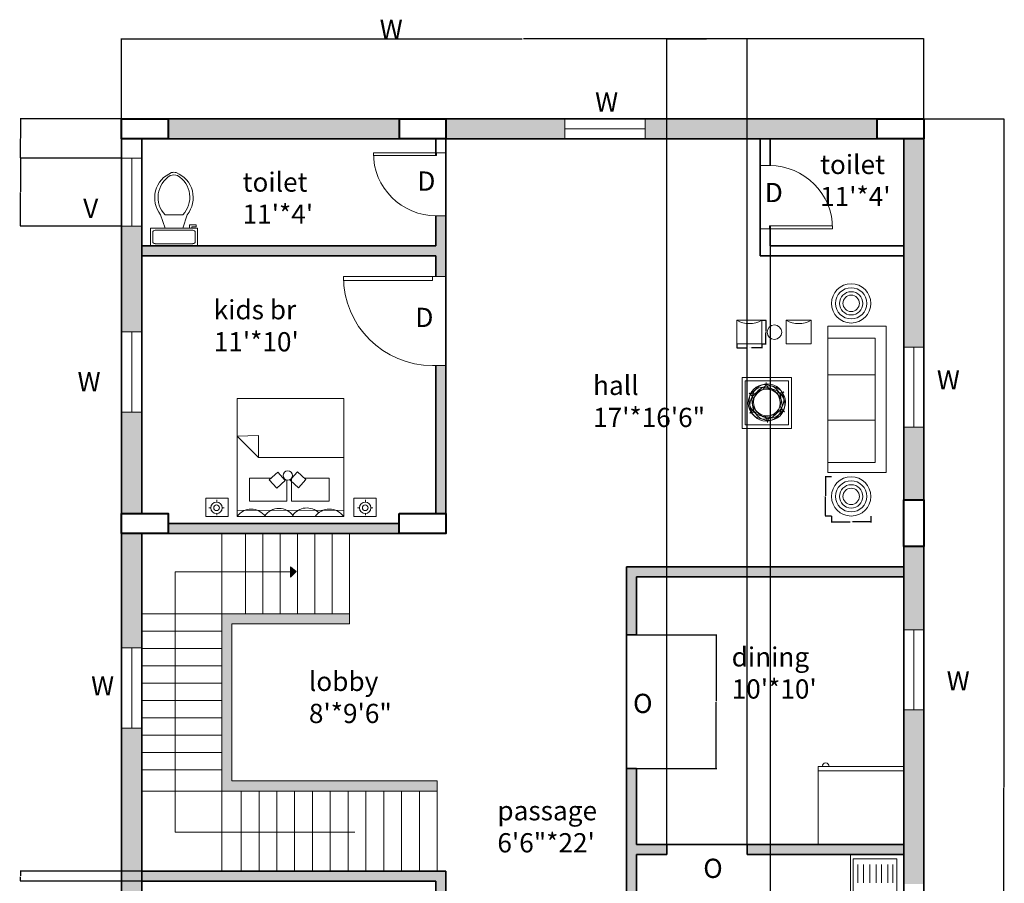
# Model space of a CAD drawing. Units: inches. Extents: x 1568 to 2529, y 2149 to 2897.
# Tile 13 of 16: x 1568 to 2010, y 2459 to 2846. Entities that reach past the tile are written whole.
import ezdxf

# ---------------------------------------------------------------- set-up
doc = ezdxf.new("R2010")
doc.units = ezdxf.units.IN
for name, color, linetype, lineweight in [('A-ANNO-DIMS', 2, 'Continuous', 18), ('A-ANNO-SYMB', 7, 'Continuous', 18), ('A-AREA-IDEN', 210, 'Continuous', 18), ('A-COLS', 7, 'Continuous', 40), ('A-DOOR', 4, 'Continuous', 18), ('A-EQPM', 8, 'Continuous', 18), ('A-FLOR-FIXT', 9, 'Continuous', 18), ('A-FLOR-STRS', 7, 'Continuous', 18), ('A-FURN', 8, 'Continuous', 18), ('A-WALL-PATT', 172, 'Continuous', 13), ('text', 210, 'Continuous', 18), ('wall', 7, 'Continuous', 35), ('window', 130, 'Continuous', 18)]:
    doc.layers.add(name, color=color, linetype=linetype, lineweight=lineweight)
doc.styles.get("Standard").update_dxf_attribs({"font": 'arial.ttf'})
doc.dimstyles.get("Standard").update_dxf_attribs({"dimtxt": 0.18, "dimasz": 0.18, "dimexe": 0.18, "dimexo": 0.0625, "dimgap": 0.09, "dimtad": 0, "dimtih": 1, "dimtoh": 1, "dimdec": 4, "dimzin": 0, "dimdsep": 46, "dimtxsty": 'Standard', "dimcen": 0.09, "dimadec": 0, "dimazin": 0, "dimtfac": 1, "dimtdec": 4, "dimtofl": 0, "dimtmove": 0, "dimatfit": 3, "dimfxl": 1, "dimtolj": 1, "dimtzin": 0, "dimarcsym": 0})

# ---------------------------------------------------------------- blocks, each defined once
blk = doc.blocks.new('*U4')
for p, q in [((9.5, -6), (9.5, -2)), ((-10, -8.5), (-8, -8.5)), ((-10, -9.5), (-10, -8.5)), ((-8, -8.5), (-8, -8)), ((-7, -8), (-7, -9.5)), ((-4, -8), (-6, -14)), ((4, -8), (6, -14)), ((-7, -9.5), (-10, -9.5)), ((4, -14), (-4, -14))]:
    blk.add_line(p, q)
blk.add_lwpolyline([(10.5, -8), (10.5, 0), (-10.5, 0), (-10.5, -8)], close=True)
for points in [[(-9.5, -2), (-9.5, -6)], [(8.5, -1), (-8.5, -1)], [(-8.5, -7), (8.5, -7)]]:
    blk.add_lwpolyline(points)
for centre, radius, start, end in [((-8.62, -1.88), 0.884, 81.8699, 188.1301), ((8.62, -1.88), 0.884, 351.8699, 98.1301), ((-8.62, -6.12), 0.884, 171.8699, 278.1301), ((8.62, -6.12), 0.884, 261.8699, 8.1301), ((3.52, -21.58), 12.17, 141.4691, 247.9714), ((4.2, -21.82), 11.33, 136.3677, 238.9468), ((-3.52, -21.58), 12.17, 292.0284, 38.5307), ((-4.2, -21.82), 11.33, 301.053, 43.6321), ((0, -27.88), 4, 245.7318, 294.2682), ((0, -29), 4, 254.8605, 285.1395)]:
    blk.add_arc(centre, radius, start, end)
blk = doc.blocks.new('*U2')
for p, q in [((0, 0), (0, -6)), ((40, 0), (40, -6))]:
    blk.add_line(p, q)
blk.add_lwpolyline([(0, 0), (0, 40), (1.75, 40), (1.75, 0)], close=True)
blk.add_arc((0, 0), 40, 0, 90)
blk = doc.blocks.new('*U5')
blk.add_circle((0, -1.46), 7.19)
for centre, start, end in [((-6.97, 10.01), 322.2254, 349.1033), ((7.14, 10.01), 190.8967, 217.7746)]:
    blk.add_arc(centre, 7.19, start, end)
blk = doc.blocks.new('*U6')
at = {"layer": 'A-FURN', "color": 0, "linetype": 'ByBlock', "lineweight": -2, "transparency": 16777216}
for p, rotation in [((1902.63, 2674.11), 59.99999999999999), ((1903.02, 2673.8), 119.9999999999999), ((1903.16, 2674.77), 300), ((1903.54, 2674.47), 240), ((1903.47, 2673.99), 180)]:
    blk.add_blockref('*U5', p, dxfattribs=dict(at, rotation=rotation))
blk.add_blockref('*U5', (1902.7, 2674.59), dxfattribs=at)
blk = doc.blocks.new('BED-WITH-NIGHTSTANDS')
for p, q in [((14.05, 36.12), (23.68, 36.4)), ((23.68, 26.45), (14.05, 36.12)), ((23.68, 36.4), (23.68, 26.45)), ((61.95, 26.45), (23.68, 26.45)), ((38.01, 16.14), (37.63, 16.49)), ((38.35, 15.84), (38.01, 16.14)), ((38.35, 16.98), (38.35, 15.84)), ((5, 6.48), (5, 7.42)), ((71.71, 6.48), (71.71, 7.42)), ((2.29, 3.95), (1.38, 3.95)), ((4.92, 1.35), (4.92, 0.55)), ((7.42, 3.92), (8.29, 3.92)), ((14.05, 2.79), (61.95, 2.73)), ((69, 3.95), (68.1, 3.95)), ((71.64, 1.35), (71.64, 0.55)), ((74.13, 3.92), (75, 3.92))]:
    blk.add_line(p, q)
for points in [[(14.05, 0), (61.95, 0), (61.95, 52.9), (14.05, 52.9)], [(31.9, 12.77), (35.7, 16.21), (32.32, 19.94), (28.52, 16.5)], [(10.04, 0), (0, 0), (0, 8.21), (10.04, 8.21)], [(76.49, 0), (66.44, 0), (66.44, 8.21), (76.49, 8.21)]]:
    blk.add_lwpolyline(points, close=True)
for points in [[(38.35, 16.98), (41.16, 20.08), (44.96, 16.64), (41.58, 12.91), (38.01, 16.14)], [(29.36, 17.26), (19.65, 17.26), (19.65, 6.93), (36.45, 6.93), (36.45, 16.34)], [(35.04, 17.26), (34.75, 17.26)], [(38.52, 17.23), (38.52, 6.93), (55.32, 6.93), (55.32, 17.26), (44.28, 17.26)], [(38.6, 17.26), (38.54, 17.26)]]:
    blk.add_lwpolyline(points)
for centre, radius in [((36.79, 18.4), 2.09), ((4.85, 3.92), 2.56), ((4.85, 3.92), 1.27), ((71.57, 3.92), 2.56), ((71.57, 3.92), 1.27)]:
    blk.add_circle(centre, radius)
for centre, start in [((20.4, -4.37), 34.5304), ((32.9, -4.09), 34.5304), ((45.42, -3.86), 46.3255), ((55.47, -4.37), 34.5304)]:
    blk.add_arc(centre, 7.71, start, 145.4696)
blk = doc.blocks.new('SOFA-THREE-SEAT')
for p, q in [((0, 60.18), (0, 65.7)), ((0, 65.7), (26.25, 65.7)), ((26.25, 65.7), (26.25, 0)), ((0, 43.78), (21.18, 43.78)), ((0, 23.43), (21.18, 23.43)), ((0, 0), (0, 5.84)), ((26.25, 0), (0, 0))]:
    blk.add_line(p, q)
blk.add_lwpolyline([(21.18, 60.18), (0, 60.18), (0, 4.48), (21.18, 4.48)], close=True)
blk = doc.blocks.new('TABLE-ROUND-END')
for radius in [8.82, 7, 5.22, 3.67]:
    blk.add_circle((0, 0), radius)
blk = doc.blocks.new('CHAIR-LOUNGE')
blk.add_lwpolyline([(0, 0), (11.26, 0), (11.26, 10.7), (0, 10.7)], close=True)
blk.add_arc((5.63, 19.97), 10.85, 238.745, 301.255)
blk = doc.blocks.new('*D19')
at = {"layer": 'A-ANNO-DIMS', "color": 0, "lineweight": -2, "transparency": 16777216}
for p, q in [((1932.04, 2641), (1929.28, 2641)), ((1929.46, 2640.82), (1929.46, 2632.37)), ((1929.46, 2623.55), (1929.46, 2632)), ((1932.04, 2623.37), (1929.28, 2623.37))]:
    blk.add_line(p, q, dxfattribs=at)
at = {"layer": 'A-ANNO-DIMS', "color": 0, "transparency": 16777216}
for points in [[(1929.43, 2640.82), (1929.49, 2640.82), (1929.46, 2641)], [(1929.43, 2623.55), (1929.49, 2623.55), (1929.46, 2623.37)]]:
    blk.add_solid(points, dxfattribs=at)
at = {"layer": 'Defpoints', "color": 0, "transparency": 16777216}
for p in [(1929.46, 2641), (1932.1, 2641), (1932.1, 2623.37)]:
    blk.add_point(p, dxfattribs=at)
at = {"layer": 'A-ANNO-DIMS', "color": 0, "transparency": 16777216, "insert": (1929.46, 2632.18), "char_height": 0.18, "attachment_point": 5}
blk.add_mtext('\\A1;END TABLE 18 TYP.', dxfattribs=at)
blk = doc.blocks.new('*D20')
at = {"layer": 'A-ANNO-DIMS', "color": 0, "lineweight": -2, "transparency": 16777216}
for p, q in [((1932.1, 2623.31), (1932.1, 2620.54)), ((1932.28, 2620.72), (1940.4, 2620.72)), ((1949.55, 2620.72), (1941.44, 2620.72)), ((1949.73, 2623.31), (1949.73, 2620.54))]:
    blk.add_line(p, q, dxfattribs=at)
at = {"layer": 'A-ANNO-DIMS', "color": 0, "transparency": 16777216}
for points in [[(1932.28, 2620.75), (1932.28, 2620.69), (1932.1, 2620.72)], [(1949.55, 2620.75), (1949.55, 2620.69), (1949.73, 2620.72)]]:
    blk.add_solid(points, dxfattribs=at)
at = {"layer": 'Defpoints', "color": 0, "transparency": 16777216}
for p in [(1932.1, 2623.37), (1932.1, 2620.72), (1949.73, 2623.37)]:
    blk.add_point(p, dxfattribs=at)
at = {"layer": 'A-ANNO-DIMS', "color": 0, "transparency": 16777216, "insert": (1940.92, 2620.72), "char_height": 0.18, "attachment_point": 5}
blk.add_mtext('\\A1;18 TYP.', dxfattribs=at)
blk = doc.blocks.new('*D23')
at = {"layer": 'A-ANNO-DIMS', "color": 0, "lineweight": -2, "transparency": 16777216}
for p, q in [((1889.61, 2700.48), (1889.61, 2698.67)), ((1900.86, 2700.48), (1900.86, 2698.67)), ((1889.79, 2698.85), (1894.28, 2698.85)), ((1900.68, 2698.85), (1896.19, 2698.85))]:
    blk.add_line(p, q, dxfattribs=at)
at = {"layer": 'A-ANNO-DIMS', "color": 0, "transparency": 16777216}
for points in [[(1889.79, 2698.88), (1889.79, 2698.82), (1889.61, 2698.85)], [(1900.68, 2698.88), (1900.68, 2698.82), (1900.86, 2698.85)]]:
    blk.add_solid(points, dxfattribs=at)
at = {"layer": 'Defpoints', "color": 0, "transparency": 16777216}
for p in [(1889.61, 2700.54), (1900.86, 2700.54), (1900.86, 2698.85)]:
    blk.add_point(p, dxfattribs=at)
at = {"layer": 'A-ANNO-DIMS', "color": 0, "transparency": 16777216, "insert": (1895.24, 2698.85), "char_height": 0.18, "attachment_point": 5}
blk.add_mtext('\\A1;CHAIR 11 TYP.', dxfattribs=at)
blk = doc.blocks.new('*D24')
at = {"layer": 'A-ANNO-DIMS', "color": 0, "lineweight": -2, "transparency": 16777216}
for p, q in [((1900.93, 2711.24), (1902.73, 2711.24)), ((1902.55, 2711.06), (1902.55, 2706.07)), ((1902.55, 2700.72), (1902.55, 2705.71)), ((1900.93, 2700.54), (1902.73, 2700.54))]:
    blk.add_line(p, q, dxfattribs=at)
at = {"layer": 'A-ANNO-DIMS', "color": 0, "transparency": 16777216}
for points in [[(1902.52, 2711.06), (1902.58, 2711.06), (1902.55, 2711.24)], [(1902.52, 2700.72), (1902.58, 2700.72), (1902.55, 2700.54)]]:
    blk.add_solid(points, dxfattribs=at)
at = {"layer": 'Defpoints', "color": 0, "transparency": 16777216}
for p in [(1900.86, 2711.24), (1902.55, 2711.24), (1900.86, 2700.54)]:
    blk.add_point(p, dxfattribs=at)
at = {"layer": 'A-ANNO-DIMS', "color": 0, "transparency": 16777216, "insert": (1902.55, 2705.89), "char_height": 0.18, "attachment_point": 5}
blk.add_mtext('\\A1;11 TYP.', dxfattribs=at)
blk = doc.blocks.new('*D27')
at = {"layer": 'A-ANNO-DIMS', "color": 0, "lineweight": -2, "transparency": 16777216}
for p, q in [((1613.55, 2801.59), (1613.55, 2837.56)), ((1613.73, 2837.38), (1793.28, 2837.38)), ((1973.4, 2837.38), (1793.85, 2837.38)), ((1973.58, 2801.59), (1973.58, 2837.56))]:
    blk.add_line(p, q, dxfattribs=at)
at = {"layer": 'A-ANNO-DIMS', "color": 0, "transparency": 16777216}
for points in [[(1613.73, 2837.41), (1613.73, 2837.35), (1613.55, 2837.38)], [(1973.4, 2837.41), (1973.4, 2837.35), (1973.58, 2837.38)]]:
    blk.add_solid(points, dxfattribs=at)
at = {"layer": 'Defpoints', "color": 0, "transparency": 16777216}
for p in [(1973.58, 2837.38), (1613.55, 2801.53), (1973.58, 2801.53)]:
    blk.add_point(p, dxfattribs=at)
at = {"layer": 'A-ANNO-DIMS', "color": 0, "transparency": 16777216, "insert": (1793.57, 2837.38), "char_height": 0.18, "attachment_point": 5}
blk.add_mtext('\\A1;360', dxfattribs=at)
blk = doc.blocks.new('*D28')
at = {"layer": 'A-ANNO-DIMS', "color": 0, "lineweight": -2, "transparency": 16777216}
for p, q in [((1973.64, 2801.53), (2009.61, 2801.53)), ((2009.43, 2801.35), (2009.43, 2501.71)), ((2009.43, 2201.71), (2009.43, 2501.35)), ((1973.61, 2201.53), (2009.61, 2201.53))]:
    blk.add_line(p, q, dxfattribs=at)
at = {"layer": 'A-ANNO-DIMS', "color": 0, "transparency": 16777216}
for points in [[(2009.4, 2801.35), (2009.46, 2801.35), (2009.43, 2801.53)], [(2009.4, 2201.71), (2009.46, 2201.71), (2009.43, 2201.53)]]:
    blk.add_solid(points, dxfattribs=at)
at = {"layer": 'Defpoints', "color": 0, "transparency": 16777216}
for p in [(1973.58, 2801.53), (2009.43, 2801.53), (1973.55, 2201.53)]:
    blk.add_point(p, dxfattribs=at)
at = {"layer": 'A-ANNO-DIMS', "color": 0, "transparency": 16777216, "insert": (2009.43, 2501.53), "char_height": 0.18, "attachment_point": 5}
blk.add_mtext('\\A1;600', dxfattribs=at)
blk = doc.blocks.new('*D32')
at = {"layer": 'A-ANNO-DIMS', "color": 0, "lineweight": -2, "transparency": 16777216}
for p, q in [((1964.55, 2792.47), (1964.55, 2165.5)), ((1904.55, 2753.4), (1904.55, 2165.5)), ((1904.73, 2165.68), (1934.33, 2165.68)), ((1964.37, 2165.68), (1934.77, 2165.68))]:
    blk.add_line(p, q, dxfattribs=at)
at = {"layer": 'A-ANNO-DIMS', "color": 0, "transparency": 16777216}
for points in [[(1904.73, 2165.71), (1904.73, 2165.65), (1904.55, 2165.68)], [(1964.37, 2165.71), (1964.37, 2165.65), (1964.55, 2165.68)]]:
    blk.add_solid(points, dxfattribs=at)
at = {"layer": 'Defpoints', "color": 0, "transparency": 16777216}
for p in [(1964.55, 2792.53), (1904.55, 2753.46), (1964.55, 2165.68)]:
    blk.add_point(p, dxfattribs=at)
at = {"layer": 'A-ANNO-DIMS', "color": 0, "transparency": 16777216, "insert": (1934.55, 2165.68), "char_height": 0.18, "attachment_point": 5}
blk.add_mtext('\\A1;60', dxfattribs=at)
blk = doc.blocks.new('*D47')
at = {"layer": 'A-ANNO-DIMS', "color": 0, "lineweight": -2, "transparency": 16777216}
for p, q in [((1622.49, 2464.03), (1567.99, 2464.03)), ((1568.17, 2463.85), (1568.17, 2461.96)), ((1568.17, 2459.71), (1568.17, 2461.6)), ((1622.49, 2459.53), (1567.99, 2459.53))]:
    blk.add_line(p, q, dxfattribs=at)
at = {"layer": 'A-ANNO-DIMS', "color": 0, "transparency": 16777216}
for points in [[(1568.14, 2463.85), (1568.2, 2463.85), (1568.17, 2464.03)], [(1568.14, 2459.71), (1568.2, 2459.71), (1568.17, 2459.53)]]:
    blk.add_solid(points, dxfattribs=at)
at = {"layer": 'Defpoints', "color": 0, "transparency": 16777216}
for p in [(1568.17, 2464.03), (1622.55, 2464.03), (1622.55, 2459.53)]:
    blk.add_point(p, dxfattribs=at)
at = {"layer": 'A-ANNO-DIMS', "color": 0, "transparency": 16777216, "insert": (1568.17, 2461.78), "char_height": 0.18, "attachment_point": 5}
blk.add_mtext('\\A1;4.5', dxfattribs=at)
blk = doc.blocks.new('*D48')
at = {"layer": 'A-ANNO-DIMS', "color": 0, "lineweight": -2, "transparency": 16777216}
for p, q in [((1844.61, 2570.08), (1880.58, 2570.08)), ((1880.4, 2569.9), (1880.4, 2540.26)), ((1880.4, 2510.26), (1880.4, 2539.89)), ((1844.61, 2510.08), (1880.58, 2510.08))]:
    blk.add_line(p, q, dxfattribs=at)
at = {"layer": 'A-ANNO-DIMS', "color": 0, "transparency": 16777216}
for points in [[(1880.37, 2569.9), (1880.43, 2569.9), (1880.4, 2570.08)], [(1880.37, 2510.26), (1880.43, 2510.26), (1880.4, 2510.08)]]:
    blk.add_solid(points, dxfattribs=at)
at = {"layer": 'Defpoints', "color": 0, "transparency": 16777216}
for p in [(1844.55, 2570.08), (1844.55, 2510.08), (1880.4, 2510.08)]:
    blk.add_point(p, dxfattribs=at)
at = {"layer": 'A-ANNO-DIMS', "color": 0, "transparency": 16777216, "insert": (1880.4, 2540.08), "char_height": 0.18, "attachment_point": 5}
blk.add_mtext('\\A1;60', dxfattribs=at)
blk = doc.blocks.new('*D49')
at = {"layer": 'A-ANNO-DIMS', "color": 0, "lineweight": -2, "transparency": 16777216}
for p, q in [((1858.18, 2476.09), (1858.18, 2837.56)), ((1858.36, 2837.38), (1875.96, 2837.38)), ((1894, 2837.38), (1876.4, 2837.38)), ((1894.18, 2476.09), (1894.18, 2837.56))]:
    blk.add_line(p, q, dxfattribs=at)
at = {"layer": 'A-ANNO-DIMS', "color": 0, "transparency": 16777216}
for points in [[(1858.36, 2837.41), (1858.36, 2837.35), (1858.18, 2837.38)], [(1894, 2837.41), (1894, 2837.35), (1894.18, 2837.38)]]:
    blk.add_solid(points, dxfattribs=at)
at = {"layer": 'Defpoints', "color": 0, "transparency": 16777216}
for p in [(1894.18, 2837.38), (1858.18, 2476.03), (1894.18, 2476.03)]:
    blk.add_point(p, dxfattribs=at)
at = {"layer": 'A-ANNO-DIMS', "color": 0, "transparency": 16777216, "insert": (1876.18, 2837.38), "char_height": 0.18, "attachment_point": 5}
blk.add_mtext('\\A1;36', dxfattribs=at)
blk = doc.blocks.new('*D50')
at = {"layer": 'A-ANNO-DIMS', "color": 0, "lineweight": -2, "transparency": 16777216}
for p, q in [((1613.49, 2783.89), (1567.99, 2783.89)), ((1568.17, 2783.71), (1568.17, 2768.8)), ((1568.17, 2753.54), (1568.17, 2768.44)), ((1613.49, 2753.36), (1567.99, 2753.36))]:
    blk.add_line(p, q, dxfattribs=at)
at = {"layer": 'A-ANNO-DIMS', "color": 0, "transparency": 16777216}
for points in [[(1568.14, 2783.71), (1568.2, 2783.71), (1568.17, 2783.89)], [(1568.14, 2753.54), (1568.2, 2753.54), (1568.17, 2753.36)]]:
    blk.add_solid(points, dxfattribs=at)
at = {"layer": 'Defpoints', "color": 0, "transparency": 16777216}
for p in [(1568.17, 2783.89), (1613.55, 2783.89), (1613.55, 2753.36)]:
    blk.add_point(p, dxfattribs=at)
at = {"layer": 'A-ANNO-DIMS', "color": 0, "transparency": 16777216, "insert": (1568.17, 2768.62), "char_height": 0.18, "attachment_point": 5}
blk.add_mtext('\\A1;30.53', dxfattribs=at)
blk = doc.blocks.new('*D51')
at = {"layer": 'A-ANNO-DIMS', "color": 0, "lineweight": -2, "transparency": 16777216}
for p, q in [((1613.49, 2801.53), (1567.99, 2801.53)), ((1568.17, 2801.35), (1568.17, 2792.89)), ((1568.17, 2784.07), (1568.17, 2792.53)), ((1613.49, 2783.89), (1567.99, 2783.89))]:
    blk.add_line(p, q, dxfattribs=at)
at = {"layer": 'A-ANNO-DIMS', "color": 0, "transparency": 16777216}
for points in [[(1568.14, 2801.35), (1568.2, 2801.35), (1568.17, 2801.53)], [(1568.14, 2784.07), (1568.2, 2784.07), (1568.17, 2783.89)]]:
    blk.add_solid(points, dxfattribs=at)
at = {"layer": 'Defpoints', "color": 0, "transparency": 16777216}
for p in [(1568.17, 2801.53), (1613.55, 2801.53), (1613.55, 2783.89)]:
    blk.add_point(p, dxfattribs=at)
at = {"layer": 'A-ANNO-DIMS', "color": 0, "transparency": 16777216, "insert": (1568.17, 2792.71), "char_height": 0.18, "attachment_point": 5}
blk.add_mtext('\\A1;17.645', dxfattribs=at)

msp = doc.modelspace()

# ---------------------------------------------------------------- hatches: boundary and pattern name
at = {"layer": 'A-ANNO-SYMB'}
h = msp.add_hatch(color=256, dxfattribs=at)
h.dxf.hatch_style = 1
h.paths.add_polyline_path([(1691.8402, 2598.4963), (1689.2797, 2600.5832), (1689.2797, 2596.9578), (1689.2797, 2595.9578)])
at = {"layer": 'A-WALL-PATT'}
h = msp.add_hatch(color=256, dxfattribs=at)
h.dxf.hatch_style = 1
h.paths.add_polyline_path([(1738.1593, 2801.532), (1634.4841, 2801.532), (1634.4841, 2792.532), (1738.1593, 2792.532)])
h.paths.add_polyline_path([(1812.4114, 2801.532), (1759.0925, 2801.532), (1759.0925, 2792.532), (1812.4114, 2792.532)])
h.paths.add_polyline_path([(1952.647, 2801.532), (1848.4114, 2801.532), (1848.4114, 2792.532), (1952.647, 2792.532)])
h.paths.add_polyline_path([(1973.5509, 2792.532), (1964.5509, 2792.532), (1964.5509, 2699.1671), (1973.5509, 2699.1671)])
h.paths.add_polyline_path([(1973.5509, 2663.1671), (1964.5509, 2663.1671), (1964.5509, 2630.5978), (1973.5509, 2630.5978)])
h.paths.add_polyline_path([(1973.5509, 2609.6646), (1964.5509, 2609.6646), (1964.5509, 2572.3679), (1973.5509, 2572.3679)])
h.paths.add_polyline_path([(1622.5509, 2753.3576), (1622.3864, 2753.3576), (1613.5509, 2753.3576), (1613.5509, 2705.9172), (1622.5509, 2705.9172)])
h.paths.add_polyline_path([(1622.5509, 2669.9172), (1613.5509, 2669.9172), (1613.5509, 2624.532), (1622.5509, 2624.532)])
h.paths.add_polyline_path([(1759.0509, 2757.9833), (1754.5509, 2757.9833), (1754.5509, 2744.532), (1622.5509, 2744.532), (1622.5509, 2740.032), (1754.5509, 2740.032), (1754.5509, 2730.8156), (1759.0509, 2730.8156), (1759.0509, 2740.032)])
h.paths.add_polyline_path([(1759.0509, 2690.8156), (1754.5509, 2690.8156), (1754.5509, 2624.532), (1759.0509, 2624.532)])
h.paths.add_polyline_path([(1738.1177, 2620.032), (1634.4841, 2620.032), (1634.4841, 2615.532), (1738.1177, 2615.532)])
h.paths.add_polyline_path([(1622.5509, 2615.532), (1613.5509, 2615.532), (1613.5509, 2564.2764), (1622.5509, 2564.2764)])
h.paths.add_polyline_path([(1759.0509, 2411.2271), (1754.5509, 2411.2271), (1754.5509, 2339.532), (1759.0509, 2339.532)])
h.paths.add_polyline_path([(1759.0509, 2464.032), (1734.3925, 2464.032), (1622.5509, 2464.032), (1622.5509, 2459.532), (1736.5509, 2459.532), (1754.5509, 2459.532), (1754.5509, 2451.2271), (1759.0509, 2451.2271)])
h.paths.add_polyline_path([(1844.5509, 2471.532), (1858.1805, 2471.532), (1858.1805, 2476.032), (1844.5509, 2476.032), (1844.5509, 2510.0763), (1840.0509, 2510.0763), (1840.0509, 2476.032), (1840.0509, 2339.532), (1844.5509, 2339.532)])
h.paths.add_polyline_path([(1844.5509, 2596.032), (1964.5509, 2596.032), (1964.5509, 2600.532), (1840.0509, 2600.532), (1840.0509, 2570.0763), (1844.5509, 2570.0763)])
h.paths.add_polyline_path([(1964.5509, 2476.032), (1894.1805, 2476.032), (1894.1805, 2471.532), (1964.5509, 2471.532)])
h.paths.add_polyline_path([(1622.5509, 2528.2764), (1613.5509, 2528.2764), (1613.5509, 2436.512), (1622.5509, 2436.512)])
h.paths.add_polyline_path([(1622.5509, 2400.512), (1613.5509, 2400.512), (1613.5509, 2339.532), (1622.5509, 2339.532)])
h.paths.add_polyline_path([(1738.9144, 2339.532), (1634.4841, 2339.532), (1634.4841, 2330.532), (1738.9144, 2330.532)])
h.paths.add_polyline_path([(1792.463, 2336.532, -0.01876983), (1792.5756, 2339.532), (1783.8928, 2339.532), (1783.8928, 2330.532), (1792.463, 2330.532)])
h.paths.add_polyline_path([(1952.6177, 2339.532), (1885.2912, 2339.532), (1885.2912, 2330.532), (1952.6177, 2330.532)])
h.paths.add_polyline_path([(1973.5509, 2422.371), (1964.5509, 2422.371), (1964.5509, 2395.032), (1964.5509, 2387.286), (1964.5509, 2339.532), (1973.5509, 2339.532)])
h.paths.add_polyline_path([(1973.5509, 2536.3679), (1964.5509, 2536.3679), (1964.5509, 2476.032), (1964.5509, 2458.371), (1973.5509, 2458.371)])
h = msp.add_hatch(color=256, dxfattribs=at)
h.dxf.hatch_style = 1
h.paths.add_polyline_path([(1715.7675, 2579.532), (1658.5509, 2579.532), (1658.5509, 2500.032), (1755.1826, 2500.032), (1755.1826, 2504.532), (1663.0509, 2504.532), (1663.0509, 2575.032), (1715.7675, 2575.032)])

# ---------------------------------------------------------------- linework, layer by layer
at = {"layer": 'A-ANNO-SYMB'}
for p, q in [((1637.5103, 2481.5328), (1637.5103, 2598.3459)), ((1637.5103, 2598.3459), (1689.2797, 2598.3459)), ((1689.2797, 2598.3459), (1689.2797, 2600.5832)), ((1689.2797, 2600.5832), (1689.2797, 2596.9578)), ((1691.8402, 2598.4963), (1689.2797, 2600.5832)), ((1689.2797, 2595.9578), (1691.8402, 2598.4963)), ((1689.2797, 2596.9578), (1689.2797, 2595.9578)), ((1718.2026, 2481.5328), (1637.5103, 2481.5328))]:
    msp.add_line(p, q, dxfattribs=at)
at = {"layer": 'A-COLS'}
for points in [[(1613.5509, 2801.532), (1634.4841, 2801.532), (1634.4841, 2792.532), (1613.5509, 2792.532)], [(1738.1593, 2801.532), (1759.0925, 2801.532), (1759.0925, 2792.532), (1738.1593, 2792.532)], [(1952.647, 2801.532), (1973.5802, 2801.532), (1973.5802, 2792.532), (1952.647, 2792.532)], [(1973.5509, 2630.5978), (1973.5509, 2609.6646), (1964.5509, 2609.6646), (1964.5509, 2630.5978)], [(1613.5509, 2624.532), (1634.4841, 2624.532), (1634.4841, 2615.532), (1613.5509, 2615.532)], [(1738.1177, 2624.532), (1759.0509, 2624.532), (1759.0509, 2615.532), (1738.1177, 2615.532)]]:
    msp.add_lwpolyline(points, close=True, dxfattribs=at)
at = {"layer": 'A-EQPM'}
msp.add_line((1964.5509, 2509.0327), (1926.0345, 2509.0327), dxfattribs=at)
for points in [[(1964.5509, 2476.032), (1926.0345, 2476.032), (1926.0345, 2510.9972), (1964.5509, 2510.9972)], [(1964.5509, 2476.032), (1964.5509, 2476.032), (1964.5509, 2476.032), (1964.5509, 2476.032)]]:
    msp.add_lwpolyline(points, close=True, dxfattribs=at)
msp.add_arc((1929.4662, 2510.9972), 1.6159, 0, 180, dxfattribs=at)
at = {"layer": 'A-FLOR-FIXT'}
for p, q in [((1964.5509, 2471.532), (1940.5509, 2471.532)), ((1940.5509, 2471.532), (1940.5509, 2339.532)), ((1943.879, 2458.902), (1943.879, 2467.0502)), ((1946.5099, 2458.902), (1946.5099, 2467.0502)), ((1949.2922, 2458.902), (1949.2922, 2467.0502)), ((1952.0744, 2458.902), (1952.0744, 2467.0502)), ((1954.5668, 2458.902), (1954.5668, 2467.0502)), ((1957.349, 2458.902), (1957.349, 2467.0502)), ((1959.6675, 2458.902), (1959.6675, 2467.0502))]:
    msp.add_line(p, q, dxfattribs=at)
msp.add_lwpolyline([(1941.7397, 2469.6671), (1961.4644, 2469.6671), (1961.4644, 2438.1142), (1941.7397, 2438.1142)], close=True, dxfattribs=at)
at = {"layer": 'A-FLOR-STRS'}
for p, q in [((1658.5509, 2579.532), (1658.5509, 2615.532)), ((1658.5509, 2615.532), (1658.5509, 2464.032)), ((1669.1171, 2615.532), (1669.1171, 2579.532)), ((1676.8922, 2615.532), (1676.8922, 2579.532)), ((1684.6673, 2615.532), (1684.6673, 2579.532)), ((1692.4423, 2615.532), (1692.4423, 2579.532)), ((1700.2174, 2615.532), (1700.2174, 2579.532)), ((1707.9924, 2615.532), (1707.9924, 2579.532)), ((1715.7675, 2615.532), (1715.7675, 2579.532)), ((1715.7675, 2575.032), (1715.7675, 2588.6853)), ((1658.5509, 2579.532), (1622.5509, 2579.532)), ((1658.5509, 2500.032), (1658.5509, 2579.532)), ((1715.7675, 2579.532), (1658.5509, 2579.532)), ((1658.5509, 2571.7569), (1622.5509, 2571.7569)), ((1715.7675, 2575.032), (1663.0509, 2575.032)), ((1663.0509, 2504.532), (1663.0509, 2575.032)), ((1658.5509, 2563.9819), (1622.5509, 2563.9819)), ((1658.5509, 2556.2068), (1622.5509, 2556.2068)), ((1658.5509, 2548.4318), (1622.5509, 2548.4318)), ((1658.5509, 2540.6567), (1622.5509, 2540.6567)), ((1658.5509, 2532.8817), (1622.5509, 2532.8817)), ((1658.5509, 2525.1066), (1622.5509, 2525.1066)), ((1658.5509, 2517.3315), (1622.5509, 2517.3315)), ((1658.5509, 2509.5565), (1622.5509, 2509.5565)), ((1755.1826, 2504.532), (1663.0509, 2504.532)), ((1755.1826, 2504.532), (1755.1826, 2490.3293)), ((1658.5509, 2500.032), (1622.5509, 2500.032)), ((1755.1826, 2500.032), (1658.5509, 2500.032)), ((1667.1826, 2464.032), (1667.1826, 2500.032)), ((1675.1826, 2464.032), (1675.1826, 2500.032)), ((1683.1826, 2464.032), (1683.1826, 2500.032)), ((1691.1826, 2464.032), (1691.1826, 2500.032)), ((1699.1826, 2464.032), (1699.1826, 2500.032)), ((1707.1826, 2464.032), (1707.1826, 2500.032)), ((1715.1826, 2464.032), (1715.1826, 2500.032)), ((1723.1826, 2464.032), (1723.1826, 2500.032)), ((1731.1826, 2464.032), (1731.1826, 2500.032)), ((1739.1826, 2464.032), (1739.1826, 2500.032)), ((1747.1826, 2464.032), (1747.1826, 2500.032)), ((1755.1826, 2464.032), (1755.1826, 2500.032)), ((1622.5509, 2464.032), (1658.5509, 2464.032))]:
    msp.add_line(p, q, dxfattribs=at)
at = {"layer": 'A-FURN'}
for points in [[(1914.1525, 2662.5617), (1892.0095, 2662.5617), (1892.0095, 2685.5203), (1914.1525, 2685.5203)], [(1912.7216, 2664.2189), (1893.4046, 2664.2189), (1893.4046, 2684.059), (1912.7216, 2684.059)]]:
    msp.add_lwpolyline(points, close=True, dxfattribs=at)
msp.add_circle((1906.4721, 2705.8298), 3.2629, dxfattribs=at)
at = {"layer": 'wall'}
for p, q in [((1622.5509, 2792.532), (1754.5509, 2792.532)), ((1754.5509, 2792.532), (1754.5509, 2785.0499)), ((1759.0509, 2792.532), (1759.0509, 2740.032)), ((1900.0509, 2792.532), (1900.0509, 2740.032)), ((1964.5509, 2792.532), (1904.5509, 2792.532)), ((1904.5509, 2792.532), (1904.5509, 2780.5289)), ((1754.5509, 2757.9844), (1754.5509, 2744.532)), ((1904.5509, 2753.4635), (1904.5509, 2744.532)), ((1754.5509, 2744.532), (1622.5509, 2744.532)), ((1904.5509, 2744.532), (1964.5509, 2744.532)), ((1754.5509, 2740.032), (1622.5509, 2740.032)), ((1754.5509, 2740.032), (1754.5509, 2730.8156)), ((1759.0509, 2740.032), (1759.0509, 2615.532)), ((1900.0509, 2740.032), (1964.5509, 2740.032)), ((1754.5509, 2690.8156), (1754.5509, 2624.532)), ((1738.1177, 2620.032), (1634.4841, 2620.032)), ((1759.0509, 2615.532), (1622.5509, 2615.532)), ((1622.5509, 2615.532), (1622.5509, 2519.532)), ((1964.5509, 2600.532), (1840.0509, 2600.532)), ((1840.0509, 2600.532), (1840.0509, 2476.032)), ((1964.5509, 2596.032), (1844.5509, 2596.032)), ((1844.5509, 2596.032), (1844.5509, 2570.0763)), ((1964.5509, 2476.032), (1964.5509, 2596.032)), ((1840.0509, 2570.0763), (1844.5509, 2570.0763)), ((1840.0509, 2510.0763), (1844.5509, 2510.0763)), ((1844.5509, 2510.0763), (1844.5509, 2476.032)), ((1840.0509, 2339.532), (1840.0509, 2476.032)), ((1844.5509, 2476.032), (1964.5509, 2476.032)), ((1858.1805, 2476.032), (1858.1805, 2471.532)), ((1894.1805, 2476.032), (1894.1805, 2471.532)), ((1844.5509, 2339.532), (1844.5509, 2471.532)), ((1844.5509, 2471.532), (1858.1805, 2471.532)), ((1894.1805, 2471.532), (1964.5509, 2471.532)), ((1622.5509, 2464.032), (1736.5509, 2464.032)), ((1759.0509, 2464.032), (1734.3925, 2464.032)), ((1759.0509, 2339.532), (1759.0509, 2464.032)), ((1622.5509, 2459.532), (1736.5509, 2459.532)), ((1622.5509, 2459.532), (1622.5509, 2339.532)), ((1754.5509, 2459.532), (1734.3925, 2459.532)), ((1754.5509, 2451.2271), (1754.5509, 2459.532))]:
    msp.add_line(p, q, dxfattribs=at)
msp.add_lwpolyline([(1613.5509, 2201.532), (1973.5509, 2201.532), (1973.5509, 2801.532), (1613.5509, 2801.532)], close=True, dxfattribs=at)
for points in [[(1964.5509, 2395.032), (1964.5509, 2792.532), (1622.5509, 2792.532), (1622.5509, 2624.532)], [(1622.5509, 2615.532), (1622.5509, 2339.532)]]:
    msp.add_lwpolyline(points, dxfattribs=at)
at = {"layer": 'window'}
for p, q in [((1812.4114, 2801.532), (1812.4114, 2792.532)), ((1848.4114, 2801.532), (1848.4114, 2792.532)), ((1812.4114, 2797.032), (1848.4114, 2797.032)), ((1613.5509, 2783.8872), (1622.5509, 2783.8872)), ((1618.0509, 2753.3576), (1618.0509, 2783.8872)), ((1613.5509, 2753.3576), (1622.4162, 2753.3576)), ((1622.3864, 2753.3576), (1622.5509, 2753.3576)), ((1613.5509, 2705.9172), (1622.5509, 2705.9172)), ((1618.0509, 2669.9172), (1618.0509, 2705.9172)), ((1964.5509, 2699.1671), (1973.5509, 2699.1671)), ((1969.0509, 2663.1671), (1969.0509, 2699.1671)), ((1613.5509, 2669.9172), (1622.5509, 2669.9172)), ((1964.5509, 2663.1671), (1973.5509, 2663.1671)), ((1964.5509, 2572.3679), (1973.5509, 2572.3679)), ((1969.0509, 2536.3679), (1969.0509, 2572.3679)), ((1613.5509, 2564.2764), (1622.5509, 2564.2764)), ((1618.0509, 2528.2764), (1618.0509, 2564.2764)), ((1964.5509, 2536.3679), (1973.5509, 2536.3679)), ((1613.5509, 2528.2764), (1622.5509, 2528.2764))]:
    msp.add_line(p, q, dxfattribs=at)

# ---------------------------------------------------------------- block references
at = {"layer": 'A-DOOR', "xscale": -0.7076230433786183, "yscale": 0.7076230433786183, "zscale": 0.7076230433786183}
for p, rotation in [((1754.8051, 2786.2882), 90), ((1904.2966, 2752.2251), 270)]:
    msp.add_blockref('*U2', p, dxfattribs=dict(at, rotation=rotation))
at = {"layer": 'A-DOOR', "xscale": -1, "rotation": 90}
msp.add_blockref('*U2', (1753.0509, 2730.8156), dxfattribs=at)
at = {"layer": 'A-FLOR-FIXT', "rotation": 180}
msp.add_blockref('*U4', (1637.0167, 2744.532), dxfattribs=at)
at = {"layer": 'A-FURN'}
for name, p in [('TABLE-ROUND-END', (1940.9182, 2718.7653)), ('CHAIR-LOUNGE', (1889.607, 2700.54)), ('CHAIR-LOUNGE', (1911.6937, 2700.54)), ('SOFA-THREE-SEAT', (1930.431, 2642.905)), ('*U6', (0, 0)), ('BED-WITH-NIGHTSTANDS', (1651.277, 2623.146))]:
    msp.add_blockref(name, p, dxfattribs=at)
at = {"layer": 'A-FURN', "rotation": 90}
msp.add_blockref('TABLE-ROUND-END', (1940.9182, 2632.1848), dxfattribs=at)

# ---------------------------------------------------------------- texts
at = {"layer": 'A-AREA-IDEN', "char_height": 8.62815, "attachment_point": 1}
for s, insert in [("toilet\\P11'*4'", (1926.9653, 2785.3778)), ("toilet\\P11'*4'", (1667.8188, 2777.4737)), ("kids br\\P11'*10'", (1654.8572, 2720.2333)), ('hall\\P17\'*16\'6"', (1825.0712, 2686.2958)), ("dining\\P10'*10'", (1887.2854, 2564.4994)), ('lobby\\P8\'*9\'6"', (1697.5703, 2553.5247)), ('passage\\P6\'6"*22\'', (1782.1432, 2495.51))]:
    msp.add_mtext_dynamic_manual_height_columns(s, width=94.297369, gutter_width=43.1407, heights=[0], dxfattribs=dict(at, insert=insert))
at = {"layer": 'text', "char_height": 8.6281, "attachment_point": 1}
for s, insert in [('W', (1729.3381, 2845.9913)), ('W', (1826.0058, 2813.3764)), ('D', (1746.2498, 2777.9089)), ('D', (1902.1481, 2772.7785)), ('V', (1596.2631, 2765.7085)), ('D', (1745.3583, 2716.771)), ('W', (1593.7523, 2687.9345)), ('W', (1979.3495, 2688.787)), ('W', (1599.8372, 2551.5157)), ('W', (1983.7718, 2553.7706)), ('O', (1843.0366, 2543.6448)), ('O', (1874.5422, 2469.6659))]:
    msp.add_mtext_dynamic_manual_height_columns(s, width=94.297369, gutter_width=43.1407, heights=[23.0437], dxfattribs=dict(at, insert=insert))

# ---------------------------------------------------------------- dimensions: what is measured, and where the dimension line sits
at = {"layer": 'A-ANNO-DIMS'}
for base, p1, p2, picture, middle in [((1973.5802, 2837.382), (1613.5509, 2801.532), (1973.5802, 2801.532), '*D27', (1793.5655, 2837.382)), ((1894.1805, 2837.382), (1858.1805, 2476.032), (1894.1805, 2476.032), '*D49', (1876.1805, 2837.382)), ((1964.5509, 2165.682), (1904.5509, 2753.4635), (1964.5509, 2792.532), '*D32', (1934.5509, 2165.682))]:
    dim = msp.add_linear_dim(base=base, p1=p1, p2=p2, dimstyle='Standard', override={"dimdec": 0, "dimlfac": 1, "dimrnd": 0, "dimzin": 0, "dimdsep": 46, "dimlunit": 2}, dxfattribs=at)
    dim.commit()
    dim.dimension.update_dxf_attribs({"geometry": picture, "text_midpoint": middle})
for base, p1, p2, angle, override, picture, middle in [((1568.1667, 2801.532), (1613.5509, 2783.8872), (1613.5509, 2801.532), 90, {"dimdec": 3, "dimlfac": 1, "dimrnd": 0, "dimzin": 0, "dimdsep": 46, "dimlunit": 2}, '*D51', (1568.1667, 2792.7096)), ((2009.4302, 2801.532), (1973.5509, 2201.532), (1973.5802, 2801.532), 90, {"dimdec": 0, "dimlfac": 1, "dimrnd": 0, "dimzin": 0, "dimdsep": 46, "dimlunit": 2}, '*D28', (2009.4302, 2501.532)), ((1568.1667, 2783.8872), (1613.5509, 2753.3576), (1613.5509, 2783.8872), 90, {"dimdec": 2, "dimlfac": 1, "dimrnd": 0, "dimzin": 0, "dimdsep": 46, "dimlunit": 2}, '*D50', (1568.1667, 2768.6224)), ((1880.4009, 2510.0763), (1844.5509, 2570.0763), (1844.5509, 2510.0763), 270, {"dimdec": 0, "dimlfac": 1, "dimrnd": 0, "dimzin": 0, "dimdsep": 46, "dimlunit": 2}, '*D48', (1880.4009, 2540.0763)), ((1568.1667, 2464.032), (1622.5509, 2459.532), (1622.5509, 2464.032), 90, {"dimdec": 1, "dimlfac": 1, "dimrnd": 0, "dimzin": 0, "dimdsep": 46, "dimlunit": 2}, '*D47', (1568.1667, 2461.782))]:
    dim = msp.add_linear_dim(base=base, p1=p1, p2=p2, angle=angle, dimstyle='Standard', override=override, dxfattribs=at)
    dim.commit()
    dim.dimension.update_dxf_attribs({"geometry": picture, "text_midpoint": middle})
for base, p1, p2, angle, text, picture, middle in [((1902.5527, 2711.2398), (1900.8641, 2700.5401), (1900.8641, 2711.2398), 90, '<> TYP.', '*D24', (1902.5527, 2705.89)), ((1929.4577, 2641.0006), (1932.1025, 2623.3691), (1932.1025, 2641.0006), 90, 'END TABLE <> TYP.', '*D19', (1929.4577, 2632.1848)), ((1932.1025, 2620.7244), (1949.734, 2623.3691), (1932.1025, 2623.3691), 180, '<> TYP.', '*D20', (1940.9182, 2620.7244))]:
    dim = msp.add_linear_dim(base=base, p1=p1, p2=p2, angle=angle, text=text, dimstyle='Standard', override={"dimdec": 0, "dimlfac": 1, "dimrnd": 0, "dimzin": 0, "dimdsep": 46, "dimlunit": 2}, dxfattribs=at)
    dim.commit()
    dim.dimension.update_dxf_attribs({"geometry": picture, "text_midpoint": middle})
dim = msp.add_linear_dim(base=(1900.8641, 2698.8515), p1=(1889.6068, 2700.5401), p2=(1900.8641, 2700.5401), text='CHAIR <> TYP.', dimstyle='Standard', override={"dimdec": 0, "dimlfac": 1, "dimrnd": 0, "dimzin": 0, "dimdsep": 46, "dimlunit": 2}, dxfattribs=at)
dim.commit()
dim.dimension.update_dxf_attribs({"geometry": '*D23', "text_midpoint": (1895.2355, 2698.8515)})

doc.saveas('drawing.dxf')
